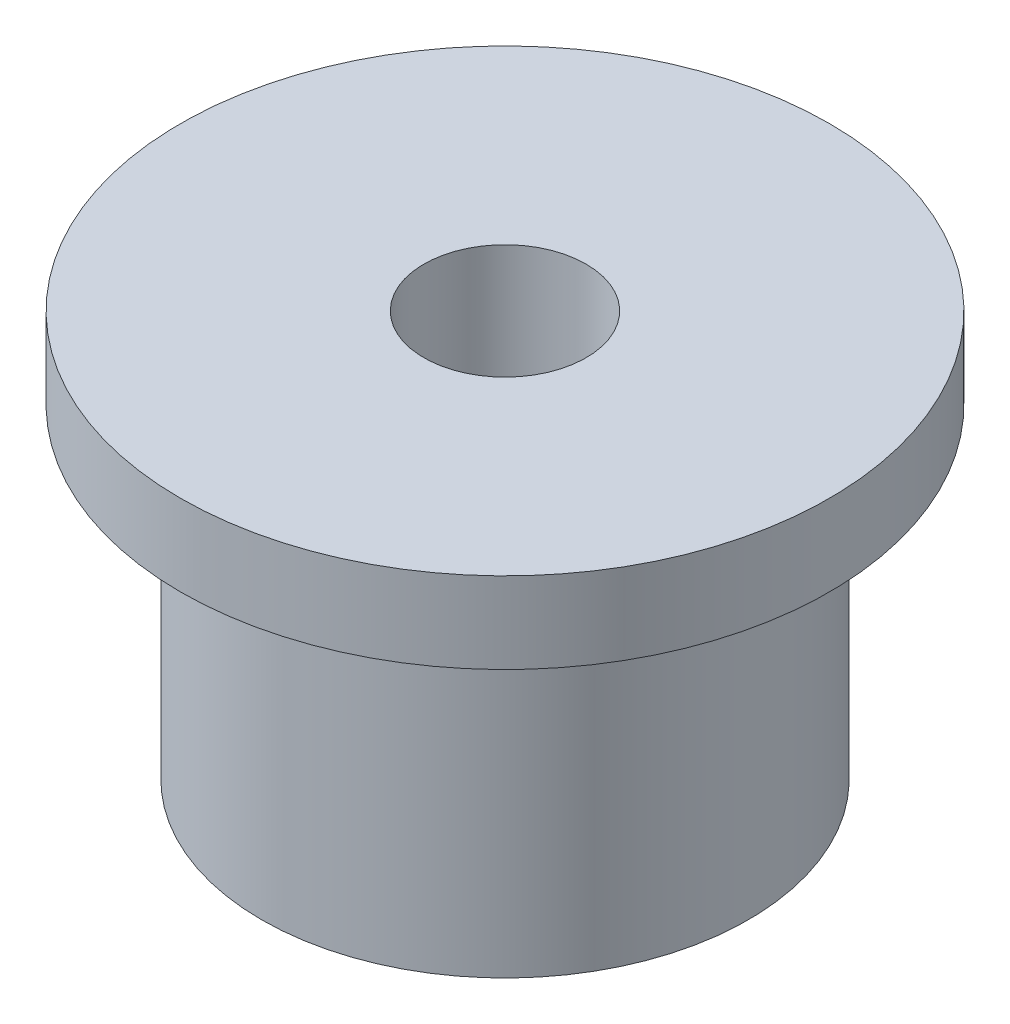
from build123d import *


with BuildPart() as part:
    # Bushing Half Profile → Flanged Bushing Revolve (revolve)
    with BuildSketch(Plane.XY, mode=Mode.PRIVATE) as flanged_bushing_revolve_sk:
        Polygon((25, 0), (25, 125), (100, 125), (100, 100), (75, 100), (75, 0), align=None)
    revolve(flanged_bushing_revolve_sk.sketch.rotate(Axis((0, 0, 0), (0, 1, 0)), 90), axis=Axis((0, 0, 0), (0, 1, 0)))


solid = part.part
